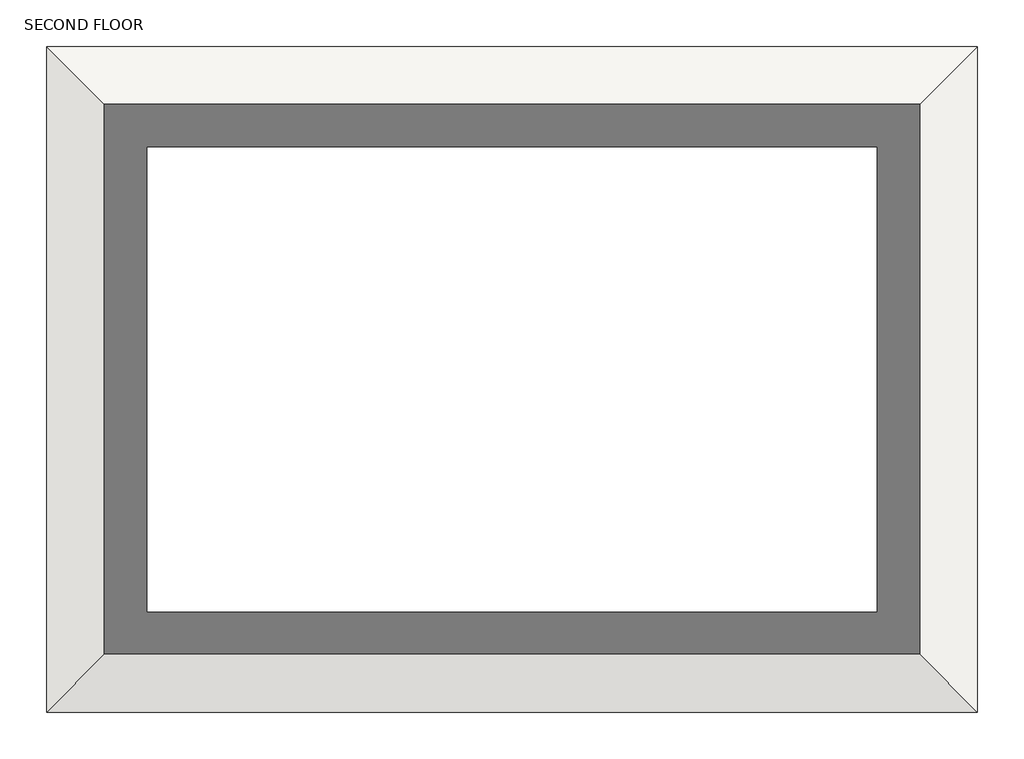
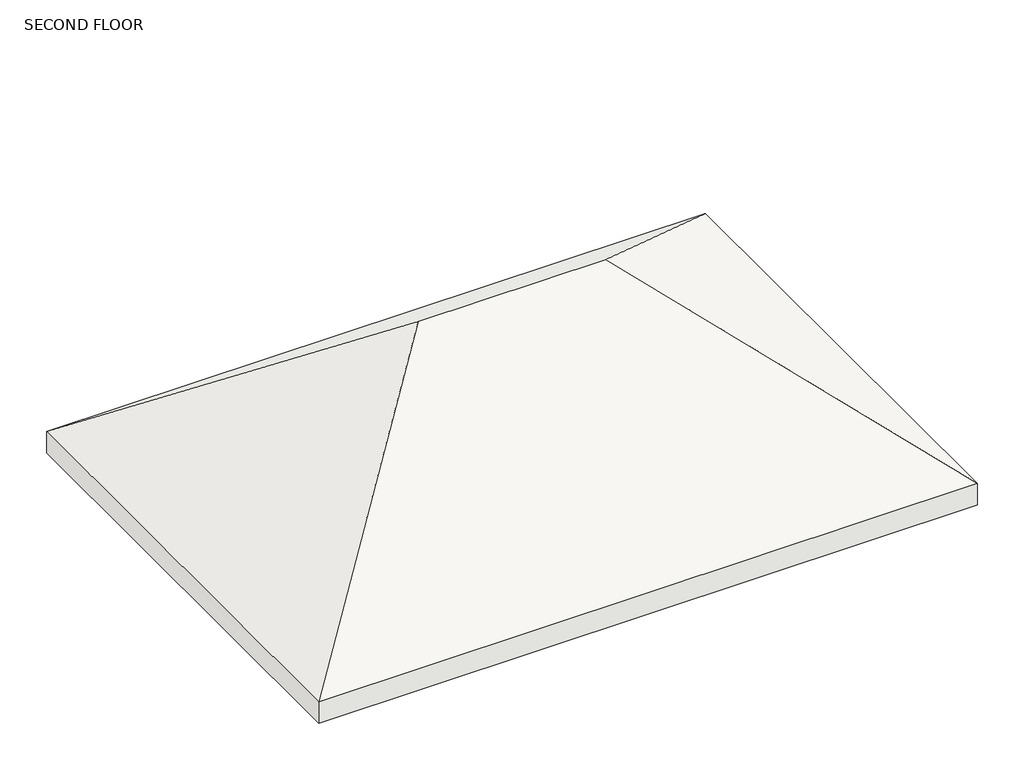
# One storey: 1 roof.
"""IFC4 building model written with IfcOpenShell, lengths in millimetres."""

from ifc_helpers import new_model, si_unit, origin, place, context, project, spatial, faceted_brep, element, save

model = new_model("IFC4")

# Units and contexts
model_context = context("Model", 3, world=origin())
ifc_project = project(units=[si_unit("LENGTHUNIT", "METRE", prefix="MILLI")], contexts=[model_context])

# Site, building, storey
site = spatial("IfcSite", under=ifc_project)
building = spatial("IfcBuilding", under=site)
storey = spatial("IfcBuildingStorey", under=building, Name="SECOND FLOOR", Elevation=7620.0)

# Roof
placement = place(None, origin())
element("IfcRoof", 1, ObjectType="Generic - 12\"", at=placement, inside=storey, context=model_context, shape_type="Brep", body=[
    faceted_brep([(1503.954407, 2797.325611, 7924.8), (-2445.745593, -1152.374389, 10887.075), (-5595.345593, -1152.374389, 10887.075), (-9545.045593, 2797.325611, 7924.8), (-9545.045593, -5102.074389, 7924.8), (1503.954407, -5102.074389, 7924.8), (1503.954407, 2797.325611, 8305.8), (-9545.045593, 2797.325611, 8305.8), (-5595.345593, -1152.374389, 11268.075), (-2445.745593, -1152.374389, 11268.075), (-9545.045593, -5102.074389, 8305.8), (1503.954407, -5102.074389, 8305.8)], [[[0, 1, 2, 3]], [[3, 2, 4]], [[4, 2, 1, 5]], [[1, 0, 5]], [[6, 7, 8, 9]], [[7, 10, 8]], [[10, 11, 9, 8]], [[6, 9, 11]], [[3, 7, 6, 0]], [[4, 10, 7, 3]], [[5, 11, 10, 4]], [[0, 6, 11, 5]]]),
])

save(model, "model.ifc")

# Revit data of these elements
# Type "Generic - 12\""
#   Assembly Code = "B1020"
#   Layers, outside or top first: 1' - 0" "ROOFING MATERIAL" (function 1)
# Element 1 (IfcRoof, "Generic - 12\"")
#   built-in parameter 1001705 = 36.9688 (stored number, unit not read)
#   built-in parameter 1001701 = 1 (stored number, unit not read)
#   built-in parameter 1001710 = 33615
#   Phase Created = New Construction
#   Materials on its faces: "ROOFING MATERIAL"
# Materials
#   "ROOFING MATERIAL": class "Generic", colour RGB 120 120 120, transparency 0, Cost = 0
